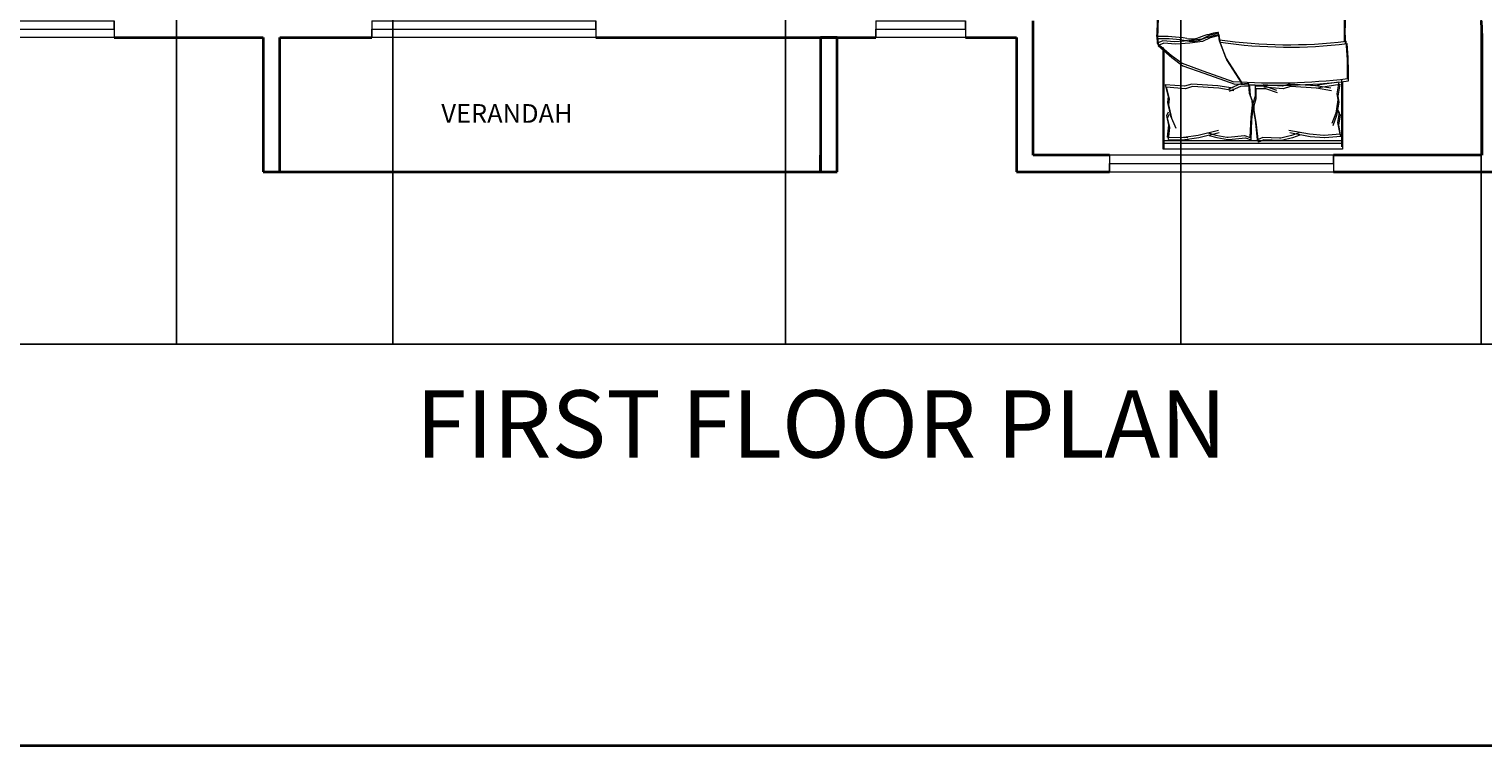
# Model space of a CAD drawing. Units: inches. Extents: x 1937 to 2996, y 1402 to 2323.
# Tile 2 of 10: x 2253 to 2643, y 1402 to 1594. Entities that reach past the tile are written whole.
import ezdxf

# ---------------------------------------------------------------- set-up
doc = ezdxf.new("R2010")
doc.units = ezdxf.units.IN
for name, color, linetype, lineweight in [('A-ANNO-DIMS', 2, 'Continuous', 18), ('A-ANNO-TTLB', 7, 'Continuous', 35), ('A-AREA-IDEN', 7, 'Continuous', 18), ('A-FURN', 8, 'Continuous', 13), ('A-GLAZ', 141, 'Continuous', 18), ('A-WALL', 7, 'Continuous', 35)]:
    doc.layers.add(name, color=color, linetype=linetype, lineweight=lineweight)
doc.styles.get("Standard").update_dxf_attribs({"font": 'arial.ttf'})
doc.dimstyles.get("Standard").update_dxf_attribs({"dimtxt": 0.18, "dimasz": 0.18, "dimexe": 0.18, "dimexo": 0.0625, "dimgap": 0.09, "dimtad": 0, "dimtih": 1, "dimtoh": 1, "dimdec": 4, "dimzin": 0, "dimdsep": 46, "dimtxsty": 'Standard', "dimcen": 0.09, "dimadec": 0, "dimazin": 0, "dimtfac": 1, "dimtdec": 4, "dimtofl": 0, "dimtmove": 0, "dimatfit": 3, "dimfxl": 1, "dimtolj": 1, "dimtzin": 0, "dimarcsym": 0})

# ---------------------------------------------------------------- blocks, each defined once
blk = doc.blocks.new('BED-DOUBLE')
for p, q in [((-24.01, -18.11), (-24.01, 0)), ((-24.01, -18.11), (-24.01, 0)), ((-24.01, 0), (24.01, 0)), ((23.78, 0), (23.78, -26.61)), ((23.78, 0), (23.78, -26.61)), ((24.01, 0), (24.01, -0.64)), ((-24.01, -1.53), (23.78, -1.53)), ((-24.01, -1.53), (23.78, -1.53)), ((-23.78, -18.75), (-23.78, -0.64)), ((-23.78, -18.75), (-23.78, -0.64)), ((-23.78, -2.17), (24.01, -2.17)), ((-23.78, -2.17), (24.01, -2.17)), ((-23.59, -3.34), (-19.3, -3.01)), ((-23.59, -3.34), (-19.31, -3.01)), ((-23.59, -3.32), (-23.01, -6.5)), ((-23.59, -3.32), (-23.01, -6.5)), ((-23.36, -3.98), (-19.08, -3.65)), ((-23.36, -3.98), (-19.08, -3.65)), ((-19.31, -3.01), (-19.2, -3.03)), ((-19.3, -3.01), (-19.2, -3.03)), ((-19.2, -3.03), (-15.38, -3.32)), ((-19.2, -3.03), (-15.38, -3.32)), ((-19.08, -3.65), (-18.97, -3.67)), ((-19.08, -3.65), (-18.97, -3.67)), ((-18.97, -3.67), (-15.15, -3.96)), ((-18.97, -3.67), (-15.15, -3.96)), ((-15.38, -3.32), (-9.88, -4.33)), ((-15.38, -3.32), (-9.88, -4.33)), ((-12.63, -3.75), (-10.61, -3.03)), ((-12.63, -3.75), (-10.61, -3.03)), ((-12.4, -4.39), (-10.38, -3.67)), ((-12.4, -4.39), (-10.38, -3.67)), ((-10.61, -3.03), (-7.71, -2.3)), ((-10.61, -3.03), (-7.71, -2.3)), ((-10.38, -3.67), (-7.49, -2.94)), ((-10.38, -3.67), (-7.49, -2.94)), ((-7.71, -2.3), (-7.39, -2.3)), ((-7.71, -2.3), (-7.39, -2.3)), ((-7.49, -2.94), (-7.16, -2.94)), ((-7.49, -2.94), (-7.16, -2.94)), ((-7.39, -2.3), (-2.95, -2.45)), ((-7.39, -2.3), (-2.95, -2.45)), ((-7.16, -2.94), (-2.72, -3.09)), ((-7.16, -2.94), (-2.72, -3.09)), ((-2.95, -2.45), (-1.5, -1.87)), ((-2.95, -2.45), (-1.5, -1.87)), ((-2.72, -3.09), (-1.27, -2.51)), ((-2.72, -3.09), (-1.27, -2.51)), ((-1.5, -1.87), (-0.92, -7.22)), ((-1.5, -1.87), (-0.92, -7.22)), ((-1.27, -2.51), (-0.7, -7.86)), ((-1.27, -2.51), (-0.7, -7.86)), ((0.49, -2.49), (0.25, -7.87)), ((0.49, -2.49), (0.25, -7.87)), ((0.72, -3.13), (0.48, -8.51)), ((0.72, -3.13), (0.48, -8.51)), ((1.97, -2.98), (0.49, -2.49)), ((1.97, -2.98), (0.49, -2.49)), ((2.2, -3.62), (0.72, -3.13)), ((2.2, -3.62), (0.72, -3.13)), ((6.4, -2.56), (1.97, -2.98)), ((6.4, -2.56), (1.97, -2.98)), ((6.63, -3.2), (2.2, -3.62)), ((6.63, -3.2), (2.2, -3.62)), ((6.72, -2.54), (6.4, -2.56)), ((6.72, -2.54), (6.4, -2.56)), ((6.95, -3.18), (6.63, -3.2)), ((6.95, -3.18), (6.63, -3.2)), ((9.65, -3.08), (6.72, -2.54)), ((9.65, -3.08), (6.72, -2.54)), ((9.88, -3.72), (6.95, -3.18)), ((9.88, -3.72), (6.95, -3.18)), ((14.43, -3.07), (9.01, -4.42)), ((14.43, -3.07), (9.01, -4.42)), ((14.66, -3.71), (9.24, -5.06)), ((14.66, -3.71), (9.24, -5.06)), ((11.72, -3.67), (9.65, -3.08)), ((11.72, -3.67), (9.65, -3.08)), ((11.94, -4.31), (9.88, -3.72)), ((11.94, -4.31), (9.88, -3.72)), ((18.23, -2.54), (14.43, -3.07)), ((18.23, -2.54), (14.43, -3.07)), ((18.46, -3.18), (14.66, -3.71)), ((18.46, -3.18), (14.66, -3.71)), ((22.63, -2.56), (17.23, -2.46)), ((17.23, -2.46), (18.23, -2.54)), ((22.63, -2.56), (17.23, -2.46)), ((17.23, -2.46), (18.23, -2.54)), ((22.86, -3.2), (17.45, -3.1)), ((17.45, -3.1), (18.46, -3.18)), ((22.86, -3.2), (17.45, -3.1)), ((17.45, -3.1), (18.46, -3.18)), ((22.63, -2.56), (22.25, -5.77)), ((22.63, -2.56), (22.25, -5.77)), ((22.86, -3.2), (22.48, -6.41)), ((22.86, -3.2), (22.48, -6.41)), ((24.01, -0.64), (24.01, -27.25)), ((24.01, -0.64), (24.01, -27.25)), ((-23.01, -6.5), (-23.45, -9.1)), ((-23.01, -6.5), (-23.45, -9.1)), ((-23.36, -3.96), (-22.78, -7.14)), ((-23.36, -3.96), (-22.78, -7.14)), ((-22.78, -7.14), (-23.22, -9.74)), ((-22.78, -7.14), (-23.22, -9.74)), ((-22.43, -8.96), (-21.42, -6.21)), ((-22.43, -8.96), (-21.42, -6.21)), ((-22.21, -9.59), (-21.19, -6.85)), ((-22.2, -9.59), (-21.19, -6.85)), ((-15.15, -3.96), (-9.65, -4.97)), ((-15.15, -3.96), (-9.65, -4.97)), ((-0.92, -7.22), (-0.35, -10.4)), ((-0.92, -7.22), (-0.35, -10.4)), ((21.83, -8.26), (20.64, -5.58)), ((21.82, -8.26), (20.64, -5.58)), ((22.05, -8.9), (20.87, -6.22)), ((22.05, -8.9), (20.87, -6.22)), ((22.25, -5.77), (22.84, -8.34)), ((22.25, -5.77), (22.84, -8.34)), ((22.48, -6.41), (23.07, -8.98)), ((22.48, -6.41), (23.07, -8.98)), ((-23.45, -9.1), (-22.87, -10.11)), ((-23.45, -9.1), (-22.87, -10.11)), ((-23.22, -9.74), (-22.64, -10.75)), ((-23.22, -9.74), (-22.64, -10.75)), ((-23.01, -12.57), (-22.43, -8.96)), ((-23.01, -12.57), (-22.43, -8.96)), ((-22.78, -13.21), (-22.2, -9.59)), ((-22.78, -13.21), (-22.21, -9.59)), ((-0.7, -7.86), (-0.12, -11.04)), ((-0.7, -7.86), (-0.12, -11.04)), ((-0.35, -10.4), (-0.35, -11.7)), ((-0.35, -10.4), (-0.35, -11.7)), ((0.25, -7.87), (-0.13, -11.08)), ((0.25, -7.87), (-0.13, -11.08)), ((-0.13, -11.08), (-0.05, -12.38)), ((-0.13, -11.08), (-0.05, -12.38)), ((-0.12, -11.04), (-0.12, -12.34)), ((-0.12, -11.04), (-0.12, -12.34)), ((0.48, -8.51), (0.1, -11.72)), ((0.48, -8.51), (0.1, -11.72)), ((22.63, -11.83), (21.82, -8.26)), ((22.63, -11.83), (21.83, -8.26)), ((22.86, -12.47), (22.05, -8.9)), ((22.86, -12.47), (22.05, -8.9)), ((22.84, -8.34), (22.33, -9.38)), ((22.84, -8.34), (22.33, -9.38)), ((23.07, -8.98), (22.56, -10.02)), ((23.07, -8.98), (22.56, -10.02)), ((-23.3, -17.34), (-22.72, -14.16)), ((-23.3, -17.34), (-22.72, -14.16)), ((-23.07, -17.98), (-22.49, -14.8)), ((-23.07, -17.98), (-22.49, -14.8)), ((-22.72, -14.16), (-23.01, -12.57)), ((-22.72, -14.16), (-23.01, -12.57)), ((-22.49, -14.8), (-22.78, -13.21)), ((-22.49, -14.8), (-22.78, -13.21)), ((-3.38, -16.26), (-6.53, -15.17)), ((-3.38, -16.26), (-6.53, -15.17)), ((-0.35, -11.7), (-0.92, -13.58)), ((-0.35, -11.7), (-0.92, -13.58)), ((-0.92, -13.58), (-0.92, -16.26)), ((-0.92, -13.58), (-0.92, -16.26)), ((-0.12, -12.34), (-0.7, -14.22)), ((-0.12, -12.34), (-0.7, -14.22)), ((-0.7, -14.22), (-0.7, -16.9)), ((-0.7, -14.22), (-0.7, -16.9)), ((-0.05, -12.38), (0.65, -14.22)), ((-0.05, -12.38), (0.65, -14.22)), ((0.1, -11.72), (0.18, -13.02)), ((0.1, -11.72), (0.18, -13.02)), ((0.18, -13.02), (0.87, -14.86)), ((0.18, -13.02), (0.87, -14.86)), ((0.65, -14.22), (0.81, -16.89)), ((0.65, -14.22), (0.81, -16.89)), ((0.87, -14.86), (1.04, -17.53)), ((0.87, -14.86), (1.04, -17.53)), ((3.27, -16.74), (6.34, -15.45)), ((3.27, -16.74), (6.34, -15.45)), ((22.44, -13.43), (22.63, -11.83)), ((22.44, -13.43), (22.63, -11.83)), ((23.21, -16.57), (22.44, -13.43)), ((23.21, -16.57), (22.44, -13.43)), ((22.67, -14.07), (22.86, -12.47)), ((22.67, -14.07), (22.86, -12.47)), ((23.44, -17.21), (22.67, -14.07)), ((23.44, -17.21), (22.67, -14.07)), ((-18.2, -16.62), (-23.3, -17.34)), ((-18.2, -16.62), (-23.3, -17.34)), ((-17.98, -17.26), (-23.07, -17.98)), ((-17.98, -17.26), (-23.07, -17.98)), ((-21.1, -15.63), (-17.07, -16.3)), ((-21.1, -15.63), (-17.07, -16.3)), ((-20.87, -16.27), (-16.84, -16.93)), ((-20.87, -16.27), (-16.84, -16.93)), ((-17.07, -16.3), (-18.2, -16.62)), ((-17.07, -16.3), (-18.2, -16.62)), ((-16.84, -16.93), (-17.98, -17.26)), ((-16.84, -16.93), (-17.98, -17.26)), ((-17.07, -16.3), (-10.06, -16.73)), ((-17.07, -16.3), (-10.06, -16.73)), ((-16.84, -16.93), (-9.83, -17.37)), ((-16.84, -16.93), (-9.83, -17.37)), ((-10.06, -16.73), (-8.1, -16.17)), ((-10.06, -16.73), (-8.1, -16.17)), ((-9.83, -17.37), (-7.87, -16.81)), ((-9.83, -17.37), (-7.87, -16.81)), ((-8.1, -16.17), (-2.97, -16.57)), ((-8.1, -16.17), (-2.97, -16.57)), ((-7.87, -16.81), (-2.74, -17.21)), ((-7.87, -16.81), (-2.74, -17.21)), ((-3.15, -16.9), (-6.3, -15.81)), ((-3.15, -16.9), (-6.3, -15.81)), ((-0.92, -16.26), (-3.38, -16.26)), ((-0.92, -16.26), (-3.38, -16.26)), ((-0.7, -16.9), (-3.15, -16.9)), ((-0.7, -16.9), (-3.15, -16.9)), ((0.81, -16.89), (3.27, -16.74)), ((0.81, -16.89), (3.27, -16.74)), ((1.04, -17.53), (3.49, -17.38)), ((1.04, -17.53), (3.49, -17.38)), ((2.77, -17.38), (6.97, -23.88)), ((2.77, -17.38), (6.96, -23.88)), ((3, -18.02), (7.19, -24.52)), ((3, -18.02), (7.19, -24.52)), ((3.49, -17.38), (6.56, -16.09)), ((3.49, -17.38), (6.56, -16.09)), ((13.16, -20.32), (4.82, -17.38)), ((13.16, -20.32), (4.82, -17.38)), ((13.39, -20.96), (5.05, -18.02)), ((13.39, -20.96), (5.05, -18.02)), ((5.08, -15.63), (9.11, -16.3)), ((5.08, -15.63), (9.11, -16.3)), ((5.31, -16.27), (9.34, -16.93)), ((5.31, -16.27), (9.34, -16.93)), ((9.11, -16.3), (16.12, -16.73)), ((9.11, -16.3), (16.12, -16.73)), ((9.34, -16.93), (16.35, -17.37)), ((9.34, -16.93), (16.35, -17.37)), ((16.12, -16.73), (18.08, -16.17)), ((16.12, -16.73), (18.08, -16.17)), ((16.35, -17.37), (18.31, -16.81)), ((16.35, -17.37), (18.31, -16.81)), ((18.08, -16.17), (23.21, -16.57)), ((18.08, -16.17), (23.21, -16.57)), ((18.31, -16.81), (23.44, -17.21)), ((18.31, -16.81), (23.44, -17.21)), ((18.74, -22.33), (13.16, -20.32)), ((18.74, -22.33), (13.16, -20.32)), ((18.96, -22.97), (13.39, -20.96)), ((18.96, -22.97), (13.39, -20.96)), ((21.68, -24.5), (18.74, -22.33)), ((21.68, -24.5), (18.74, -22.33)), ((21.91, -25.13), (18.96, -22.97)), ((21.91, -25.13), (18.96, -22.97)), ((6.96, -23.88), (8.67, -28.37)), ((6.97, -23.88), (8.67, -28.37)), ((7.19, -24.52), (8.9, -29)), ((7.19, -24.52), (8.9, -29)), ((25.38, -27.75), (21.68, -24.5)), ((25.38, -27.75), (21.68, -24.5)), ((25.61, -28.39), (21.91, -25.13)), ((25.61, -28.39), (21.91, -25.13)), ((8.67, -28.37), (8.98, -30.38)), ((8.67, -28.37), (8.98, -30.38)), ((8.9, -29), (9.21, -31.02)), ((8.9, -29), (9.21, -31.02)), ((8.98, -30.38), (11.46, -29.76)), ((8.98, -30.38), (11.46, -29.76)), ((9.21, -31.02), (11.68, -30.4)), ((9.21, -31.02), (11.68, -30.4)), ((11.46, -29.76), (13.47, -28.83)), ((11.46, -29.76), (13.47, -28.83)), ((11.68, -30.4), (13.7, -29.47)), ((11.68, -30.4), (13.7, -29.47)), ((13.47, -28.83), (16.88, -28.37)), ((13.47, -28.83), (16.88, -28.37)), ((13.7, -29.47), (17.11, -29)), ((13.7, -29.47), (17.1, -29)), ((16.88, -28.37), (20.75, -28.06)), ((16.88, -28.37), (20.75, -28.06)), ((17.1, -29), (20.98, -28.69)), ((17.11, -29), (20.98, -28.69)), ((20.75, -28.06), (23.85, -28.37)), ((20.75, -28.06), (23.85, -28.37)), ((20.98, -28.69), (24.07, -29)), ((20.98, -28.69), (24.07, -29)), ((23.85, -28.37), (25.38, -27.75)), ((23.85, -28.37), (25.38, -27.75)), ((24.07, -29), (25.61, -28.39)), ((24.07, -29), (25.61, -28.39)), ((25.46, -29.49), (25.38, -27.75, 3.87)), ((25.46, -29.49), (25.38, -27.75, 3.87)), ((25.69, -30.13), (25.61, -28.39, 3.87)), ((25.69, -30.13), (25.61, -28.39, 3.87)), ((-12.42, -79.25), (12.19, -79.25)), ((-12.42, -79.25), (12.19, -79.25)), ((-12.19, -79.88), (12.42, -79.88)), ((-12.19, -79.88), (12.42, -79.88))]:
    blk.add_line(p, q)
for centre, radius, start, end in [((57.68, -20.1), 83.31, 178.7218, 185.604), ((57.68, -20.1), 83.31, 178.7218, 185.604), ((-6.13, -182.05), 164.97, 86.0865, 96.7821), ((-6.13, -182.05), 164.97, 86.0865, 96.7821), ((57.91, -20.74), 83.31, 178.7218, 185.604), ((57.91, -20.74), 83.31, 178.7218, 185.604), ((-5.9, -182.69), 164.97, 86.0865, 96.7821), ((-5.9, -182.69), 164.97, 86.0865, 96.7821), ((-9.73, -156.32), 129.02, 81.7845, 96.9006), ((-9.73, -156.32), 129.02, 81.7845, 96.9006), ((-9.5, -156.96), 129.02, 81.7845, 96.9006), ((-9.5, -156.96), 129.02, 81.7845, 96.9006), ((-194.79, -31.17), 170.11, 358.4762, 1.0082), ((-194.79, -31.17), 170.11, 358.4762, 1.0082), ((-194.56, -31.81), 170.11, 358.4762, 1.0082), ((-194.56, -31.81), 170.11, 358.4762, 1.0082), ((9.15, -30.44), 0.185, 160.2464, 271.1377), ((9.15, -30.44), 0.185, 160.2464, 271.1377), ((3.67, -1.48), 29.65, 280.6617, 289.8806), ((3.67, -1.48), 29.65, 280.6617, 289.8806), ((9.38, -31.08), 0.185, 160.2464, 271.1377), ((9.38, -31.08), 0.185, 160.2464, 271.1377), ((3.9, -2.12), 29.65, 280.6617, 289.8806), ((3.9, -2.12), 29.65, 280.6617, 289.8806), ((16.26, -35.07), 6.22, 78.6608, 113.7384), ((16.26, -35.07), 6.22, 78.6608, 113.7384), ((16.49, -35.71), 6.22, 78.6608, 113.7384), ((16.49, -35.71), 6.22, 78.6608, 113.7384), ((23.84, 6.66), 36.18, 259.8763, 272.5657), ((23.84, 6.66), 36.18, 259.8763, 272.5657), ((24.07, 6.02), 36.18, 259.8763, 272.5657), ((24.07, 6.02), 36.18, 259.8763, 272.5657), ((154.78, -36.32), 129.5, 176.9791, 183.8365), ((154.78, -36.32), 129.5, 176.9791, 183.8365), ((155.01, -36.95), 129.5, 176.9791, 183.8365), ((155.01, -36.95), 129.5, 176.9791, 183.8365), ((457.34, -50.61), 482.31, 178.2277, 181.7185), ((457.34, -50.61), 482.31, 178.2277, 181.7185), ((457.57, -51.25), 482.31, 178.2277, 181.7185), ((457.57, -51.25), 482.31, 178.2277, 181.7185), ((-4536.23, -67.82), 4561.86, 0.00217, 0.28689), ((-4536.23, -67.82), 4561.86, 0.00217, 0.28689), ((-4536, -68.46), 4561.86, 0.00217, 0.28689), ((-4536, -68.46), 4561.86, 0.00217, 0.28689), ((-54.38, -64.52), 29.63, 346.0648, 358.9113), ((-54.38, -64.52), 29.63, 346.0648, 358.9113), ((-54.16, -65.15), 29.63, 346.0648, 358.9113), ((-54.16, -65.15), 29.63, 346.0648, 358.9113), ((48.67, -68.67), 23.07, 177.4714, 206.4681), ((48.67, -68.67), 23.07, 177.4714, 206.4681), ((48.9, -69.31), 23.07, 177.4714, 206.4681), ((48.9, -69.31), 23.07, 177.4714, 206.4681), ((-49.14, -70.28), 23.56, 337.9751, 356.652), ((-49.14, -70.28), 23.56, 337.9751, 356.652), ((-48.92, -70.91), 23.56, 337.9751, 356.652), ((-48.92, -70.91), 23.56, 337.9751, 356.652), ((-44.71, 23.71), 106.46, 283.3832, 287.7053), ((-44.71, 23.71), 106.46, 283.3832, 287.7053), ((-26.4, -79.72), 1.09, 146.1736, 293.4781), ((-26.4, -79.72), 1.09, 146.1736, 293.4781), ((-26.17, -80.36), 1.09, 146.1736, 293.4781), ((-26.17, -80.36), 1.09, 146.1736, 293.4781), ((-6.06, -200.84), 121.76, 92.9958, 99.4091), ((-6.06, -200.84), 121.76, 92.9958, 99.4091), ((-5.83, -201.48), 121.76, 92.9958, 99.4091), ((-5.83, -201.48), 121.76, 92.9958, 99.4091), ((-44.48, 23.07), 106.46, 283.3832, 287.7053), ((-44.48, 23.07), 106.46, 283.3832, 287.7053), ((13.67, -212.28), 133.04, 84.4998, 90.6351), ((13.67, -212.28), 133.04, 84.4998, 90.6351), ((13.9, -212.92), 133.04, 84.4998, 90.6351), ((13.9, -212.92), 133.04, 84.4998, 90.6351), ((26.93, -78.87), 1.1, 242.6588, 356.02), ((26.93, -78.87), 1.1, 242.6588, 356.02), ((27.15, -79.51), 1.1, 242.6588, 356.02), ((27.15, -79.51), 1.1, 242.6588, 356.02)]:
    blk.add_arc(centre, radius, start, end)
blk = doc.blocks.new('WINDOW-60IN')
for p, q in [((0, 2.25), (0, -2.25)), ((0, 2.25), (60, 2.25)), ((0, -2.25), (0, 0)), ((0, 0), (60, 0)), ((60, 0), (60, 2.25)), ((60, 2.25), (60, -2.25)), ((60, -2.25), (0, -2.25))]:
    blk.add_line(p, q)
blk = doc.blocks.new('WINDOW-24IN')
for p, q in [((0, -2.25), (0, 2.25)), ((0, 2.25), (0, 0)), ((24, 2.25), (0, 2.25)), ((0, 0), (24, 0)), ((24, -2.25), (24, 2.25)), ((24, 0), (24, -2.25)), ((0, -2.25), (24, -2.25))]:
    blk.add_line(p, q)
blk = doc.blocks.new('WINDOW-36IN')
for p, q in [((0, 2.25), (0, -2.25)), ((0, 2.25), (36, 2.25)), ((36, 0), (36, 2.25)), ((36, 2.25), (36, -2.25)), ((0, -2.25), (0, 0)), ((0, 0), (36, 0)), ((36, -2.25), (0, -2.25))]:
    blk.add_line(p, q)
blk = doc.blocks.new('*D23')
at = {"layer": 'A-ANNO-DIMS', "color": 0, "lineweight": -2, "transparency": 16777216}
for p, q in [((2010.65, 1769.24), (2010.65, 1508.98)), ((2924.15, 1769.24), (2924.15, 1508.98)), ((2010.83, 1509.16), (2467, 1509.16)), ((2923.97, 1509.16), (2467.79, 1509.16))]:
    blk.add_line(p, q, dxfattribs=at)
at = {"layer": 'A-ANNO-DIMS', "color": 0, "transparency": 16777216}
for points in [[(2010.83, 1509.19), (2010.83, 1509.13), (2010.65, 1509.16)], [(2923.97, 1509.19), (2923.97, 1509.13), (2924.15, 1509.16)]]:
    blk.add_solid(points, dxfattribs=at)
at = {"layer": 'Defpoints', "color": 0, "transparency": 16777216}
for p in [(2010.65, 1769.31), (2924.15, 1769.31), (2924.15, 1509.16)]:
    blk.add_point(p, dxfattribs=at)
at = {"layer": 'A-ANNO-DIMS', "color": 0, "transparency": 16777216, "insert": (2467.4, 1509.16), "char_height": 0.18, "attachment_point": 5}
blk.add_mtext('\\A1;913.5', dxfattribs=at)
blk = doc.blocks.new('*D33')
at = {"layer": 'A-ANNO-DIMS', "color": 0, "lineweight": -2, "transparency": 16777216}
for p, q in [((2292.65, 1849.24), (2292.65, 1508.98)), ((2350.61, 1849.24), (2350.61, 1508.98)), ((2292.83, 1509.16), (2321.24, 1509.16)), ((2350.43, 1509.16), (2322.02, 1509.16))]:
    blk.add_line(p, q, dxfattribs=at)
at = {"layer": 'A-ANNO-DIMS', "color": 0, "transparency": 16777216}
for points in [[(2292.83, 1509.19), (2292.83, 1509.13), (2292.65, 1509.16)], [(2350.43, 1509.19), (2350.43, 1509.13), (2350.61, 1509.16)]]:
    blk.add_solid(points, dxfattribs=at)
at = {"layer": 'Defpoints', "color": 0, "transparency": 16777216}
for p in [(2292.65, 1849.31), (2350.61, 1849.31), (2350.61, 1509.16)]:
    blk.add_point(p, dxfattribs=at)
at = {"layer": 'A-ANNO-DIMS', "color": 0, "transparency": 16777216, "insert": (2321.63, 1509.16), "char_height": 0.18, "attachment_point": 5}
blk.add_mtext('\\A1;57.96', dxfattribs=at)
blk = doc.blocks.new('*D34')
at = {"layer": 'A-ANNO-DIMS', "color": 0, "lineweight": -2, "transparency": 16777216}
for p, q in [((2350.61, 1849.24), (2350.61, 1508.98)), ((2561.65, 1849.24), (2561.65, 1508.98)), ((2350.79, 1509.16), (2455.66, 1509.16)), ((2561.47, 1509.16), (2456.59, 1509.16))]:
    blk.add_line(p, q, dxfattribs=at)
at = {"layer": 'A-ANNO-DIMS', "color": 0, "transparency": 16777216}
for points in [[(2350.79, 1509.19), (2350.79, 1509.13), (2350.61, 1509.16)], [(2561.47, 1509.19), (2561.47, 1509.13), (2561.65, 1509.16)]]:
    blk.add_solid(points, dxfattribs=at)
at = {"layer": 'Defpoints', "color": 0, "transparency": 16777216}
for p in [(2350.61, 1849.31), (2561.65, 1849.31), (2561.65, 1509.16)]:
    blk.add_point(p, dxfattribs=at)
at = {"layer": 'A-ANNO-DIMS', "color": 0, "transparency": 16777216, "insert": (2456.13, 1509.16), "char_height": 0.18, "attachment_point": 5}
blk.add_mtext('\\A1;211.04', dxfattribs=at)
blk = doc.blocks.new('*D35')
at = {"layer": 'A-ANNO-DIMS', "color": 0, "lineweight": -2, "transparency": 16777216}
for p, q in [((2561.65, 1849.24), (2561.65, 1508.98)), ((2642.15, 1849.24), (2642.15, 1508.98)), ((2561.83, 1509.16), (2601.57, 1509.16)), ((2641.97, 1509.16), (2602.22, 1509.16))]:
    blk.add_line(p, q, dxfattribs=at)
at = {"layer": 'A-ANNO-DIMS', "color": 0, "transparency": 16777216}
for points in [[(2561.83, 1509.19), (2561.83, 1509.13), (2561.65, 1509.16)], [(2641.97, 1509.19), (2641.97, 1509.13), (2642.15, 1509.16)]]:
    blk.add_solid(points, dxfattribs=at)
at = {"layer": 'Defpoints', "color": 0, "transparency": 16777216}
for p in [(2561.65, 1849.31), (2642.15, 1849.31), (2642.15, 1509.16)]:
    blk.add_point(p, dxfattribs=at)
at = {"layer": 'A-ANNO-DIMS', "color": 0, "transparency": 16777216, "insert": (2601.9, 1509.16), "char_height": 0.18, "attachment_point": 5}
blk.add_mtext('\\A1;80.5', dxfattribs=at)
blk = doc.blocks.new('*D38')
at = {"layer": 'A-ANNO-DIMS', "color": 0, "lineweight": -2, "transparency": 16777216}
for p, q in [((2350.61, 1895.99), (2350.61, 1508.98)), ((2455.77, 1895.99), (2455.77, 1508.98)), ((2350.79, 1509.16), (2402.74, 1509.16)), ((2455.59, 1509.16), (2403.65, 1509.16))]:
    blk.add_line(p, q, dxfattribs=at)
at = {"layer": 'A-ANNO-DIMS', "color": 0, "transparency": 16777216}
for points in [[(2350.79, 1509.19), (2350.79, 1509.13), (2350.61, 1509.16)], [(2455.59, 1509.19), (2455.59, 1509.13), (2455.77, 1509.16)]]:
    blk.add_solid(points, dxfattribs=at)
at = {"layer": 'Defpoints', "color": 0, "transparency": 16777216}
for p in [(2350.61, 1896.06), (2455.77, 1896.06), (2455.77, 1509.16)]:
    blk.add_point(p, dxfattribs=at)
at = {"layer": 'A-ANNO-DIMS', "color": 0, "transparency": 16777216, "insert": (2403.19, 1509.16), "char_height": 0.18, "attachment_point": 5}
blk.add_mtext('\\A1;105.16', dxfattribs=at)

msp = doc.modelspace()

# ---------------------------------------------------------------- linework, layer by layer
at = {"layer": 'A-ANNO-TTLB'}
msp.add_lwpolyline([(1937.1125, 2323.2883), (2995.8132, 2323.2883), (2995.8132, 1401.6335), (1937.1125, 1401.6335)], close=True, dxfattribs=at)
at = {"layer": 'A-GLAZ'}
for p, q in [((2602.6116, 1559.8061), (2542.5478, 1559.8061)), ((2542.6116, 1559.8061), (2542.6116, 1555.3061)), ((2602.6116, 1557.5561), (2602.6116, 1559.8061)), ((2602.6116, 1559.8061), (2602.6116, 1555.3061)), ((2542.6116, 1555.3061), (2542.6116, 1557.5561)), ((2542.6116, 1557.5561), (2602.6116, 1557.5561)), ((2542.6116, 1555.3061), (2602.6116, 1555.3061))]:
    msp.add_line(p, q, dxfattribs=at)
at = {"layer": 'A-WALL'}
for p, q in [((2522.1473, 1559.8061), (2522.1473, 1595.8061)), ((2642.1473, 1595.8061), (2642.2867, 1591.3061)), ((2275.9586, 1591.3061), (2315.8789, 1591.3061)), ((2315.8789, 1591.3061), (2315.8789, 1555.3061)), ((2320.3789, 1555.3061), (2320.3789, 1591.3061)), ((2320.3789, 1591.3061), (2321.1473, 1591.3061)), ((2321.1473, 1591.3061), (2344.9752, 1591.3061)), ((2404.9752, 1591.3061), (2480.0063, 1591.3061)), ((2469.6473, 1591.3061), (2465.1473, 1591.3061)), ((2465.1473, 1591.3061), (2465.1473, 1555.3061)), ((2469.6473, 1555.3061), (2469.6473, 1591.3061)), ((2504.0063, 1591.3061), (2517.6473, 1591.3061)), ((2517.6473, 1591.3061), (2517.6473, 1555.3061)), ((2642.2867, 1591.3061), (2642.2867, 1559.8061)), ((2465.1473, 1555.3061), (2465.1473, 1559.8061)), ((2542.6116, 1559.8061), (2522.1473, 1559.8061)), ((2642.2867, 1559.8061), (2602.6116, 1559.8061)), ((2315.8789, 1555.3061), (2469.6473, 1555.3061)), ((2517.6473, 1555.3061), (2542.6116, 1555.3061)), ((2602.6116, 1555.3061), (2646.6473, 1555.3061))]:
    msp.add_line(p, q, dxfattribs=at)

# ---------------------------------------------------------------- block references
at = {"layer": 'A-FURN', "rotation": 180}
msp.add_blockref('BED-DOUBLE', (2580.9749, 1561.4249), dxfattribs=at)
at = {"layer": 'A-GLAZ'}
for name, p in [('WINDOW-36IN', (2239.9586, 1593.5561)), ('WINDOW-60IN', (2344.9752, 1593.5561))]:
    msp.add_blockref(name, p, dxfattribs=at)
at = {"layer": 'A-GLAZ', "extrusion": (0, 0, -1), "zscale": -1, "rotation": 180}
msp.add_blockref('WINDOW-24IN', (-2480.0063, 1593.5561), dxfattribs=at)

# ---------------------------------------------------------------- texts
at = {"layer": 'A-ANNO-TTLB', "insert": (2356.7664, 1496.846), "char_height": 18, "attachment_point": 1}
msp.add_mtext_dynamic_manual_height_columns('FIRST FLOOR PLAN', width=1058.562847, gutter_width=12.5, heights=[0], dxfattribs=at)
at = {"layer": 'A-AREA-IDEN', "insert": (2363.6178, 1573.4698), "char_height": 5, "attachment_point": 1}
msp.add_mtext_dynamic_manual_height_columns('VERANDAH', width=137.071433, gutter_width=12.5, heights=[0], dxfattribs=at)

# ---------------------------------------------------------------- dimensions: what is measured, and where the dimension line sits
at = {"layer": 'A-ANNO-DIMS'}
for base, p1, p2, override, picture, middle in [((2455.7744, 1509.1561), (2350.6104, 1896.0561), (2455.7744, 1896.0561), {"dimdec": 2, "dimlfac": 1, "dimrnd": 0, "dimzin": 0, "dimdsep": 46, "dimlunit": 2}, '*D38', (2403.1924, 1509.1561)), ((2350.6104, 1509.1561), (2292.6473, 1849.3061), (2350.6104, 1849.3061), {"dimdec": 2, "dimlfac": 1, "dimrnd": 0, "dimzin": 0, "dimdsep": 46, "dimlunit": 2}, '*D33', (2321.6289, 1509.1561)), ((2561.6473, 1509.1561), (2350.6104, 1849.3061), (2561.6473, 1849.3061), {"dimdec": 2, "dimlfac": 1, "dimrnd": 0, "dimzin": 0, "dimdsep": 46, "dimlunit": 2}, '*D34', (2456.1289, 1509.1561)), ((2642.1473, 1509.1561), (2561.6473, 1849.3061), (2642.1473, 1849.3061), {"dimdec": 1, "dimlfac": 1, "dimrnd": 0, "dimzin": 0, "dimdsep": 46, "dimlunit": 2}, '*D35', (2601.8973, 1509.1561)), ((2924.1473, 1509.1561), (2010.6473, 1769.3061), (2924.1473, 1769.3061), {"dimdec": 1, "dimlfac": 1, "dimrnd": 0, "dimzin": 0, "dimdsep": 46, "dimlunit": 2}, '*D23', (2467.3973, 1509.1561))]:
    dim = msp.add_linear_dim(base=base, p1=p1, p2=p2, dimstyle='Standard', override=override, dxfattribs=at)
    dim.commit()
    dim.dimension.update_dxf_attribs({"geometry": picture, "text_midpoint": middle})

doc.saveas('drawing.dxf')
